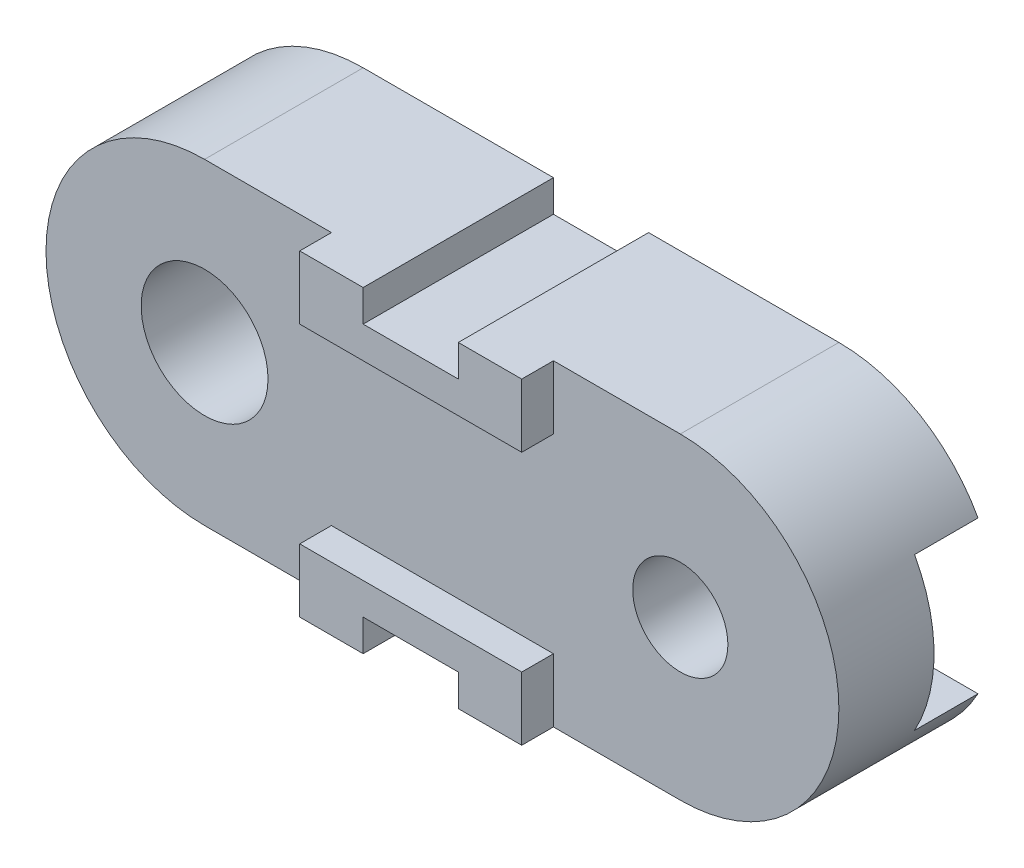
ISO-10303-21;
HEADER;
FILE_DESCRIPTION(('STEP AP214'),'2;1');
FILE_NAME('part.step','',(''),(''),'','','');
FILE_SCHEMA(('AUTOMOTIVE_DESIGN { 1 0 10303 214 1 1 1 1 }'));
ENDSEC;
DATA;
#1=APPLICATION_CONTEXT('core data for automotive mechanical design processes');
#2=APPLICATION_PROTOCOL_DEFINITION('international standard','automotive_design',2000,#1);
#3=PRODUCT_CONTEXT('',#1,'mechanical');
#4=PRODUCT('Part','Part','',(#3));
#5=PRODUCT_RELATED_PRODUCT_CATEGORY('part','',(#4));
#6=PRODUCT_DEFINITION_FORMATION('','',#4);
#7=PRODUCT_DEFINITION_CONTEXT('part definition',#1,'design');
#8=PRODUCT_DEFINITION('design','',#6,#7);
#9=PRODUCT_DEFINITION_SHAPE('','',#8);
#10=(LENGTH_UNIT() NAMED_UNIT(*) SI_UNIT(.MILLI.,.METRE.));
#11=(NAMED_UNIT(*) PLANE_ANGLE_UNIT() SI_UNIT($,.RADIAN.));
#12=(NAMED_UNIT(*) SI_UNIT($,.STERADIAN.) SOLID_ANGLE_UNIT());
#13=UNCERTAINTY_MEASURE_WITH_UNIT(LENGTH_MEASURE(1.E-05),#10,'distance_accuracy_value','');
#14=(GEOMETRIC_REPRESENTATION_CONTEXT(3) GLOBAL_UNCERTAINTY_ASSIGNED_CONTEXT((#13)) GLOBAL_UNIT_ASSIGNED_CONTEXT((#10,
#11,#12)) REPRESENTATION_CONTEXT('',''));
#15=CARTESIAN_POINT('',(0.,0.,0.));
#16=DIRECTION('',(0.,0.,1.));
#17=DIRECTION('',(1.,0.,0.));
#18=AXIS2_PLACEMENT_3D('',#15,#16,#17);
#19=CARTESIAN_POINT('',(-37.5,-25.,25.));
#20=DIRECTION('',(0.,1.,0.));
#21=DIRECTION('',(-1.,0.,0.));
#22=AXIS2_PLACEMENT_3D('',#19,#20,#21);
#23=PLANE('',#22);
#24=DIRECTION('',(1.,0.,0.));
#25=VECTOR('',#24,1.);
#26=CARTESIAN_POINT('',(17.5,-25.,30.));
#27=LINE('',#26,#25);
#28=CARTESIAN_POINT('',(7.5,-25.,30.));
#29=VERTEX_POINT('',#28);
#30=CARTESIAN_POINT('',(17.5,-25.,30.));
#31=VERTEX_POINT('',#30);
#32=EDGE_CURVE('E327',#29,#31,#27,.T.);
#33=ORIENTED_EDGE('',*,*,#32,.F.);
#34=DIRECTION('',(0.,0.,-1.));
#35=VECTOR('',#34,1.);
#36=CARTESIAN_POINT('',(7.5,-25.,25.));
#37=LINE('',#36,#35);
#38=CARTESIAN_POINT('',(7.5,-25.,0.));
#39=VERTEX_POINT('',#38);
#40=EDGE_CURVE('E281',#29,#39,#37,.T.);
#41=ORIENTED_EDGE('',*,*,#40,.T.);
#42=DIRECTION('',(1.,0.,0.));
#43=VECTOR('',#42,1.);
#44=CARTESIAN_POINT('',(-37.5,-25.,0.));
#45=LINE('',#44,#43);
#46=CARTESIAN_POINT('',(37.5,-25.,0.));
#47=VERTEX_POINT('',#46);
#48=EDGE_CURVE('E367',#39,#47,#45,.T.);
#49=ORIENTED_EDGE('',*,*,#48,.T.);
#50=DIRECTION('',(0.,0.,-1.));
#51=VECTOR('',#50,1.);
#52=CARTESIAN_POINT('',(37.5,-25.,25.));
#53=LINE('',#52,#51);
#54=CARTESIAN_POINT('',(37.5,-25.,25.));
#55=VERTEX_POINT('',#54);
#56=EDGE_CURVE('E387',#55,#47,#53,.T.);
#57=ORIENTED_EDGE('',*,*,#56,.F.);
#58=DIRECTION('',(1.,0.,0.));
#59=VECTOR('',#58,1.);
#60=CARTESIAN_POINT('',(-37.5,-25.,25.));
#61=LINE('',#60,#59);
#62=CARTESIAN_POINT('',(17.5,-25.,25.));
#63=VERTEX_POINT('',#62);
#64=EDGE_CURVE('E357',#63,#55,#61,.T.);
#65=ORIENTED_EDGE('',*,*,#64,.F.);
#66=DIRECTION('',(0.,0.,-1.));
#67=VECTOR('',#66,1.);
#68=CARTESIAN_POINT('',(17.5,-25.,30.));
#69=LINE('',#68,#67);
#70=EDGE_CURVE('E344',#31,#63,#69,.T.);
#71=ORIENTED_EDGE('',*,*,#70,.F.);
#72=EDGE_LOOP('',(#33,#41,#49,#57,#65,#71));
#73=FACE_BOUND('',#72,.T.);
#74=ADVANCED_FACE('F44',(#73),#23,.F.);
#75=CARTESIAN_POINT('',(-37.5,25.,25.));
#76=DIRECTION('',(0.,-1.,0.));
#77=DIRECTION('',(1.,0.,0.));
#78=AXIS2_PLACEMENT_3D('',#75,#76,#77);
#79=PLANE('',#78);
#80=DIRECTION('',(-1.,0.,0.));
#81=VECTOR('',#80,1.);
#82=CARTESIAN_POINT('',(17.5,25.,30.));
#83=LINE('',#82,#81);
#84=CARTESIAN_POINT('',(-7.5,25.,30.));
#85=VERTEX_POINT('',#84);
#86=CARTESIAN_POINT('',(-17.5,25.,30.));
#87=VERTEX_POINT('',#86);
#88=EDGE_CURVE('E296',#85,#87,#83,.T.);
#89=ORIENTED_EDGE('',*,*,#88,.F.);
#90=DIRECTION('',(0.,0.,-1.));
#91=VECTOR('',#90,1.);
#92=CARTESIAN_POINT('',(-7.5,25.,25.));
#93=LINE('',#92,#91);
#94=CARTESIAN_POINT('',(-7.5,25.,0.));
#95=VERTEX_POINT('',#94);
#96=EDGE_CURVE('E271',#85,#95,#93,.T.);
#97=ORIENTED_EDGE('',*,*,#96,.T.);
#98=DIRECTION('',(-1.,0.,0.));
#99=VECTOR('',#98,1.);
#100=CARTESIAN_POINT('',(-37.5,25.,0.));
#101=LINE('',#100,#99);
#102=CARTESIAN_POINT('',(-37.5,25.,0.));
#103=VERTEX_POINT('',#102);
#104=EDGE_CURVE('E378',#95,#103,#101,.T.);
#105=ORIENTED_EDGE('',*,*,#104,.T.);
#106=DIRECTION('',(0.,0.,-1.));
#107=VECTOR('',#106,1.);
#108=CARTESIAN_POINT('',(-37.5,25.,25.));
#109=LINE('',#108,#107);
#110=CARTESIAN_POINT('',(-37.5,25.,25.));
#111=VERTEX_POINT('',#110);
#112=EDGE_CURVE('E370',#111,#103,#109,.T.);
#113=ORIENTED_EDGE('',*,*,#112,.F.);
#114=DIRECTION('',(-1.,0.,0.));
#115=VECTOR('',#114,1.);
#116=CARTESIAN_POINT('',(-37.5,25.,25.));
#117=LINE('',#116,#115);
#118=CARTESIAN_POINT('',(-17.5,25.,25.));
#119=VERTEX_POINT('',#118);
#120=EDGE_CURVE('E365',#119,#111,#117,.T.);
#121=ORIENTED_EDGE('',*,*,#120,.F.);
#122=DIRECTION('',(0.,0.,-1.));
#123=VECTOR('',#122,1.);
#124=CARTESIAN_POINT('',(-17.5,25.,30.));
#125=LINE('',#124,#123);
#126=EDGE_CURVE('E305',#87,#119,#125,.T.);
#127=ORIENTED_EDGE('',*,*,#126,.F.);
#128=EDGE_LOOP('',(#89,#97,#105,#113,#121,#127));
#129=FACE_BOUND('',#128,.T.);
#130=ADVANCED_FACE('F417',(#129),#79,.F.);
#131=CARTESIAN_POINT('',(-37.5,0.,25.));
#132=DIRECTION('',(0.,0.,1.));
#133=DIRECTION('',(1.,0.,0.));
#134=AXIS2_PLACEMENT_3D('',#131,#132,#133);
#135=PLANE('',#134);
#136=CARTESIAN_POINT('',(37.5,0.,25.));
#137=DIRECTION('',(0.,0.,1.));
#138=DIRECTION('',(1.,0.,0.));
#139=AXIS2_PLACEMENT_3D('',#136,#137,#138);
#140=CIRCLE('',#139,7.5);
#141=CARTESIAN_POINT('',(45.,0.,25.));
#142=VERTEX_POINT('',#141);
#143=EDGE_CURVE('E408',#142,#142,#140,.T.);
#144=ORIENTED_EDGE('',*,*,#143,.F.);
#145=EDGE_LOOP('',(#144));
#146=FACE_BOUND('',#145,.T.);
#147=CARTESIAN_POINT('',(-37.5,0.,25.));
#148=DIRECTION('',(0.,0.,1.));
#149=DIRECTION('',(1.,0.,0.));
#150=AXIS2_PLACEMENT_3D('',#147,#148,#149);
#151=CIRCLE('',#150,10.);
#152=CARTESIAN_POINT('',(-27.5,0.,25.));
#153=VERTEX_POINT('',#152);
#154=EDGE_CURVE('E235',#153,#153,#151,.T.);
#155=ORIENTED_EDGE('',*,*,#154,.F.);
#156=EDGE_LOOP('',(#155));
#157=FACE_BOUND('',#156,.T.);
#158=DIRECTION('',(1.,0.,0.));
#159=VECTOR('',#158,1.);
#160=CARTESIAN_POINT('',(0.,15.,25.));
#161=LINE('',#160,#159);
#162=CARTESIAN_POINT('',(-17.5,15.,25.));
#163=VERTEX_POINT('',#162);
#164=CARTESIAN_POINT('',(17.5,15.,25.));
#165=VERTEX_POINT('',#164);
#166=EDGE_CURVE('E304',#163,#165,#161,.T.);
#167=ORIENTED_EDGE('',*,*,#166,.F.);
#168=DIRECTION('',(0.,-1.,0.));
#169=VECTOR('',#168,1.);
#170=CARTESIAN_POINT('',(-17.5,25.,25.));
#171=LINE('',#170,#169);
#172=EDGE_CURVE('E288',#119,#163,#171,.T.);
#173=ORIENTED_EDGE('',*,*,#172,.F.);
#174=ORIENTED_EDGE('',*,*,#120,.T.);
#175=CARTESIAN_POINT('',(-37.5,0.,25.));
#176=DIRECTION('',(0.,0.,1.));
#177=DIRECTION('',(1.,0.,0.));
#178=AXIS2_PLACEMENT_3D('',#175,#176,#177);
#179=CIRCLE('',#178,25.);
#180=CARTESIAN_POINT('',(-37.5,-25.,25.));
#181=VERTEX_POINT('',#180);
#182=EDGE_CURVE('E354',#111,#181,#179,.T.);
#183=ORIENTED_EDGE('',*,*,#182,.T.);
#184=CARTESIAN_POINT('',(-17.5,-25.,25.));
#185=VERTEX_POINT('',#184);
#186=EDGE_CURVE('E359',#181,#185,#61,.T.);
#187=ORIENTED_EDGE('',*,*,#186,.T.);
#188=DIRECTION('',(0.,-1.,0.));
#189=VECTOR('',#188,1.);
#190=CARTESIAN_POINT('',(-17.5,-25.,25.));
#191=LINE('',#190,#189);
#192=CARTESIAN_POINT('',(-17.5,-15.,25.));
#193=VERTEX_POINT('',#192);
#194=EDGE_CURVE('E321',#193,#185,#191,.T.);
#195=ORIENTED_EDGE('',*,*,#194,.F.);
#196=DIRECTION('',(-1.,0.,0.));
#197=VECTOR('',#196,1.);
#198=CARTESIAN_POINT('',(0.,-15.,25.));
#199=LINE('',#198,#197);
#200=CARTESIAN_POINT('',(17.5,-15.,25.));
#201=VERTEX_POINT('',#200);
#202=EDGE_CURVE('E326',#201,#193,#199,.T.);
#203=ORIENTED_EDGE('',*,*,#202,.F.);
#204=DIRECTION('',(0.,1.,0.));
#205=VECTOR('',#204,1.);
#206=CARTESIAN_POINT('',(17.5,-15.,25.));
#207=LINE('',#206,#205);
#208=EDGE_CURVE('E336',#63,#201,#207,.T.);
#209=ORIENTED_EDGE('',*,*,#208,.F.);
#210=ORIENTED_EDGE('',*,*,#64,.T.);
#211=CARTESIAN_POINT('',(37.5,0.,25.));
#212=DIRECTION('',(0.,0.,1.));
#213=DIRECTION('',(1.,0.,0.));
#214=AXIS2_PLACEMENT_3D('',#211,#212,#213);
#215=CIRCLE('',#214,25.);
#216=CARTESIAN_POINT('',(37.5,25.,25.));
#217=VERTEX_POINT('',#216);
#218=EDGE_CURVE('E362',#55,#217,#215,.T.);
#219=ORIENTED_EDGE('',*,*,#218,.T.);
#220=CARTESIAN_POINT('',(17.5,25.,25.));
#221=VERTEX_POINT('',#220);
#222=EDGE_CURVE('E364',#217,#221,#117,.T.);
#223=ORIENTED_EDGE('',*,*,#222,.T.);
#224=DIRECTION('',(0.,1.,0.));
#225=VECTOR('',#224,1.);
#226=CARTESIAN_POINT('',(17.5,15.,25.));
#227=LINE('',#226,#225);
#228=EDGE_CURVE('E294',#165,#221,#227,.T.);
#229=ORIENTED_EDGE('',*,*,#228,.F.);
#230=EDGE_LOOP('',(#167,#173,#174,#183,#187,#195,#203,#209,#210,#219,#223,#229));
#231=FACE_BOUND('',#230,.T.);
#232=ADVANCED_FACE('F413',(#146,#157,#231),#135,.T.);
#233=CARTESIAN_POINT('',(-37.5,0.,25.));
#234=DIRECTION('',(0.,0.,-1.));
#235=DIRECTION('',(-1.,0.,0.));
#236=AXIS2_PLACEMENT_3D('',#233,#234,#235);
#237=CYLINDRICAL_SURFACE('',#236,25.);
#238=CARTESIAN_POINT('',(-37.5,0.,0.));
#239=DIRECTION('',(0.,0.,1.));
#240=DIRECTION('',(1.,0.,0.));
#241=AXIS2_PLACEMENT_3D('',#238,#239,#240);
#242=CIRCLE('',#241,25.);
#243=CARTESIAN_POINT('',(-37.5,-25.,0.));
#244=VERTEX_POINT('',#243);
#245=EDGE_CURVE('E352',#103,#244,#242,.T.);
#246=ORIENTED_EDGE('',*,*,#245,.T.);
#247=DIRECTION('',(0.,0.,-1.));
#248=VECTOR('',#247,1.);
#249=CARTESIAN_POINT('',(-37.5,-25.,25.));
#250=LINE('',#249,#248);
#251=EDGE_CURVE('E386',#181,#244,#250,.T.);
#252=ORIENTED_EDGE('',*,*,#251,.F.);
#253=ORIENTED_EDGE('',*,*,#182,.F.);
#254=ORIENTED_EDGE('',*,*,#112,.T.);
#255=EDGE_LOOP('',(#246,#252,#253,#254));
#256=FACE_BOUND('',#255,.T.);
#257=ADVANCED_FACE('F50',(#256),#237,.T.);
#258=CARTESIAN_POINT('',(-7.5,-25.,0.));
#259=VERTEX_POINT('',#258);
#260=EDGE_CURVE('E371',#244,#259,#45,.T.);
#261=ORIENTED_EDGE('',*,*,#260,.T.);
#262=DIRECTION('',(0.,0.,1.));
#263=VECTOR('',#262,1.);
#264=CARTESIAN_POINT('',(-7.5,-25.,25.));
#265=LINE('',#264,#263);
#266=CARTESIAN_POINT('',(-7.5,-25.,30.));
#267=VERTEX_POINT('',#266);
#268=EDGE_CURVE('E280',#259,#267,#265,.T.);
#269=ORIENTED_EDGE('',*,*,#268,.T.);
#270=CARTESIAN_POINT('',(-17.5,-25.,30.));
#271=VERTEX_POINT('',#270);
#272=EDGE_CURVE('E328',#271,#267,#27,.T.);
#273=ORIENTED_EDGE('',*,*,#272,.F.);
#274=DIRECTION('',(0.,0.,-1.));
#275=VECTOR('',#274,1.);
#276=CARTESIAN_POINT('',(-17.5,-25.,30.));
#277=LINE('',#276,#275);
#278=EDGE_CURVE('E346',#271,#185,#277,.T.);
#279=ORIENTED_EDGE('',*,*,#278,.T.);
#280=ORIENTED_EDGE('',*,*,#186,.F.);
#281=ORIENTED_EDGE('',*,*,#251,.T.);
#282=EDGE_LOOP('',(#261,#269,#273,#279,#280,#281));
#283=FACE_BOUND('',#282,.T.);
#284=ADVANCED_FACE('F440',(#283),#23,.F.);
#285=CARTESIAN_POINT('',(37.5,0.,25.));
#286=DIRECTION('',(0.,0.,-1.));
#287=DIRECTION('',(-1.,0.,0.));
#288=AXIS2_PLACEMENT_3D('',#285,#286,#287);
#289=CYLINDRICAL_SURFACE('',#288,25.);
#290=CARTESIAN_POINT('',(37.5,0.,0.));
#291=DIRECTION('',(0.,0.,1.));
#292=DIRECTION('',(1.,0.,0.));
#293=AXIS2_PLACEMENT_3D('',#290,#291,#292);
#294=CIRCLE('',#293,25.);
#295=CARTESIAN_POINT('',(59.4317121994613,-12.,0.));
#296=VERTEX_POINT('',#295);
#297=EDGE_CURVE('E374',#47,#296,#294,.T.);
#298=ORIENTED_EDGE('',*,*,#297,.T.);
#299=DIRECTION('',(0.,0.,-1.));
#300=VECTOR('',#299,1.);
#301=CARTESIAN_POINT('',(59.4317121994613,-12.,25.));
#302=LINE('',#301,#300);
#303=CARTESIAN_POINT('',(59.4317121994613,-12.,10.));
#304=VERTEX_POINT('',#303);
#305=EDGE_CURVE('E238',#296,#304,#302,.F.);
#306=ORIENTED_EDGE('',*,*,#305,.T.);
#307=CARTESIAN_POINT('',(37.5,0.,10.));
#308=DIRECTION('',(0.,0.,-1.));
#309=DIRECTION('',(-1.,0.,0.));
#310=AXIS2_PLACEMENT_3D('',#307,#308,#309);
#311=CIRCLE('',#310,25.);
#312=CARTESIAN_POINT('',(59.4317121994613,12.,10.));
#313=VERTEX_POINT('',#312);
#314=EDGE_CURVE('E11',#313,#304,#311,.T.);
#315=ORIENTED_EDGE('',*,*,#314,.F.);
#316=DIRECTION('',(0.,0.,-1.));
#317=VECTOR('',#316,1.);
#318=CARTESIAN_POINT('',(59.4317121994613,12.,25.));
#319=LINE('',#318,#317);
#320=CARTESIAN_POINT('',(59.4317121994613,12.,0.));
#321=VERTEX_POINT('',#320);
#322=EDGE_CURVE('E222',#313,#321,#319,.T.);
#323=ORIENTED_EDGE('',*,*,#322,.T.);
#324=CARTESIAN_POINT('',(37.5,25.,0.));
#325=VERTEX_POINT('',#324);
#326=EDGE_CURVE('E372',#321,#325,#294,.T.);
#327=ORIENTED_EDGE('',*,*,#326,.T.);
#328=DIRECTION('',(0.,0.,-1.));
#329=VECTOR('',#328,1.);
#330=CARTESIAN_POINT('',(37.5,25.,25.));
#331=LINE('',#330,#329);
#332=EDGE_CURVE('E382',#217,#325,#331,.T.);
#333=ORIENTED_EDGE('',*,*,#332,.F.);
#334=ORIENTED_EDGE('',*,*,#218,.F.);
#335=ORIENTED_EDGE('',*,*,#56,.T.);
#336=EDGE_LOOP('',(#298,#306,#315,#323,#327,#333,#334,#335));
#337=FACE_BOUND('',#336,.T.);
#338=ADVANCED_FACE('F459',(#337),#289,.T.);
#339=CARTESIAN_POINT('',(7.5,25.,0.));
#340=VERTEX_POINT('',#339);
#341=EDGE_CURVE('E358',#325,#340,#101,.T.);
#342=ORIENTED_EDGE('',*,*,#341,.T.);
#343=DIRECTION('',(0.,0.,1.));
#344=VECTOR('',#343,1.);
#345=CARTESIAN_POINT('',(7.5,25.,25.));
#346=LINE('',#345,#344);
#347=CARTESIAN_POINT('',(7.5,25.,30.));
#348=VERTEX_POINT('',#347);
#349=EDGE_CURVE('E264',#340,#348,#346,.T.);
#350=ORIENTED_EDGE('',*,*,#349,.T.);
#351=CARTESIAN_POINT('',(17.5,25.,30.));
#352=VERTEX_POINT('',#351);
#353=EDGE_CURVE('E297',#352,#348,#83,.T.);
#354=ORIENTED_EDGE('',*,*,#353,.F.);
#355=DIRECTION('',(0.,0.,-1.));
#356=VECTOR('',#355,1.);
#357=CARTESIAN_POINT('',(17.5,25.,30.));
#358=LINE('',#357,#356);
#359=EDGE_CURVE('E315',#352,#221,#358,.T.);
#360=ORIENTED_EDGE('',*,*,#359,.T.);
#361=ORIENTED_EDGE('',*,*,#222,.F.);
#362=ORIENTED_EDGE('',*,*,#332,.T.);
#363=EDGE_LOOP('',(#342,#350,#354,#360,#361,#362));
#364=FACE_BOUND('',#363,.T.);
#365=ADVANCED_FACE('F470',(#364),#79,.F.);
#366=CARTESIAN_POINT('',(-37.5,0.,0.));
#367=DIRECTION('',(0.,0.,1.));
#368=DIRECTION('',(1.,0.,0.));
#369=AXIS2_PLACEMENT_3D('',#366,#367,#368);
#370=PLANE('',#369);
#371=CARTESIAN_POINT('',(-37.5,0.,0.));
#372=DIRECTION('',(0.,0.,1.));
#373=DIRECTION('',(1.,0.,0.));
#374=AXIS2_PLACEMENT_3D('',#371,#372,#373);
#375=CIRCLE('',#374,10.);
#376=CARTESIAN_POINT('',(-27.5,0.,0.));
#377=VERTEX_POINT('',#376);
#378=EDGE_CURVE('E237',#377,#377,#375,.T.);
#379=ORIENTED_EDGE('',*,*,#378,.T.);
#380=EDGE_LOOP('',(#379));
#381=FACE_BOUND('',#380,.T.);
#382=CARTESIAN_POINT('',(37.5,0.,0.));
#383=DIRECTION('',(0.,0.,-1.));
#384=DIRECTION('',(-1.,0.,0.));
#385=AXIS2_PLACEMENT_3D('',#382,#383,#384);
#386=CIRCLE('',#385,12.);
#387=CARTESIAN_POINT('',(37.5,-12.,0.));
#388=VERTEX_POINT('',#387);
#389=CARTESIAN_POINT('',(37.5,12.,0.));
#390=VERTEX_POINT('',#389);
#391=EDGE_CURVE('E65',#388,#390,#386,.T.);
#392=ORIENTED_EDGE('',*,*,#391,.F.);
#393=DIRECTION('',(1.,0.,0.));
#394=VECTOR('',#393,1.);
#395=CARTESIAN_POINT('',(-37.5,-12.,0.));
#396=LINE('',#395,#394);
#397=EDGE_CURVE('E53',#388,#296,#396,.T.);
#398=ORIENTED_EDGE('',*,*,#397,.T.);
#399=ORIENTED_EDGE('',*,*,#297,.F.);
#400=ORIENTED_EDGE('',*,*,#48,.F.);
#401=DIRECTION('',(0.,1.,0.));
#402=VECTOR('',#401,1.);
#403=CARTESIAN_POINT('',(7.5,0.,0.));
#404=LINE('',#403,#402);
#405=CARTESIAN_POINT('',(7.5,-20.,0.));
#406=VERTEX_POINT('',#405);
#407=EDGE_CURVE('E278',#39,#406,#404,.T.);
#408=ORIENTED_EDGE('',*,*,#407,.T.);
#409=DIRECTION('',(-1.,0.,0.));
#410=VECTOR('',#409,1.);
#411=CARTESIAN_POINT('',(-37.5,-20.,0.));
#412=LINE('',#411,#410);
#413=CARTESIAN_POINT('',(-7.5,-20.,0.));
#414=VERTEX_POINT('',#413);
#415=EDGE_CURVE('E286',#406,#414,#412,.T.);
#416=ORIENTED_EDGE('',*,*,#415,.T.);
#417=DIRECTION('',(0.,-1.,0.));
#418=VECTOR('',#417,1.);
#419=CARTESIAN_POINT('',(-7.5,0.,0.));
#420=LINE('',#419,#418);
#421=EDGE_CURVE('E273',#414,#259,#420,.T.);
#422=ORIENTED_EDGE('',*,*,#421,.T.);
#423=ORIENTED_EDGE('',*,*,#260,.F.);
#424=ORIENTED_EDGE('',*,*,#245,.F.);
#425=ORIENTED_EDGE('',*,*,#104,.F.);
#426=DIRECTION('',(0.,-1.,0.));
#427=VECTOR('',#426,1.);
#428=CARTESIAN_POINT('',(-7.5,0.,0.));
#429=LINE('',#428,#427);
#430=CARTESIAN_POINT('',(-7.5,20.,0.));
#431=VERTEX_POINT('',#430);
#432=EDGE_CURVE('E268',#95,#431,#429,.T.);
#433=ORIENTED_EDGE('',*,*,#432,.T.);
#434=DIRECTION('',(1.,0.,0.));
#435=VECTOR('',#434,1.);
#436=CARTESIAN_POINT('',(-37.5,20.,0.));
#437=LINE('',#436,#435);
#438=CARTESIAN_POINT('',(7.5,20.,0.));
#439=VERTEX_POINT('',#438);
#440=EDGE_CURVE('E253',#431,#439,#437,.T.);
#441=ORIENTED_EDGE('',*,*,#440,.T.);
#442=DIRECTION('',(0.,1.,0.));
#443=VECTOR('',#442,1.);
#444=CARTESIAN_POINT('',(7.5,0.,0.));
#445=LINE('',#444,#443);
#446=EDGE_CURVE('E265',#439,#340,#445,.T.);
#447=ORIENTED_EDGE('',*,*,#446,.T.);
#448=ORIENTED_EDGE('',*,*,#341,.F.);
#449=ORIENTED_EDGE('',*,*,#326,.F.);
#450=DIRECTION('',(1.,0.,0.));
#451=VECTOR('',#450,1.);
#452=CARTESIAN_POINT('',(37.5,12.,0.));
#453=LINE('',#452,#451);
#454=EDGE_CURVE('E226',#390,#321,#453,.T.);
#455=ORIENTED_EDGE('',*,*,#454,.F.);
#456=EDGE_LOOP('',(#392,#398,#399,#400,#408,#416,#422,#423,#424,#425,#433,#441,#447,#448,#449,#455));
#457=FACE_BOUND('',#456,.T.);
#458=ADVANCED_FACE('F476',(#381,#457),#370,.F.);
#459=CARTESIAN_POINT('',(-17.5,-25.,30.));
#460=DIRECTION('',(1.,0.,0.));
#461=DIRECTION('',(0.,0.,-1.));
#462=AXIS2_PLACEMENT_3D('',#459,#460,#461);
#463=PLANE('',#462);
#464=ORIENTED_EDGE('',*,*,#194,.T.);
#465=ORIENTED_EDGE('',*,*,#278,.F.);
#466=DIRECTION('',(0.,-1.,0.));
#467=VECTOR('',#466,1.);
#468=CARTESIAN_POINT('',(-17.5,-25.,30.));
#469=LINE('',#468,#467);
#470=CARTESIAN_POINT('',(-17.5,-15.,30.));
#471=VERTEX_POINT('',#470);
#472=EDGE_CURVE('E324',#471,#271,#469,.T.);
#473=ORIENTED_EDGE('',*,*,#472,.F.);
#474=DIRECTION('',(0.,0.,-1.));
#475=VECTOR('',#474,1.);
#476=CARTESIAN_POINT('',(-17.5,-15.,30.));
#477=LINE('',#476,#475);
#478=EDGE_CURVE('E353',#471,#193,#477,.T.);
#479=ORIENTED_EDGE('',*,*,#478,.T.);
#480=EDGE_LOOP('',(#464,#465,#473,#479));
#481=FACE_BOUND('',#480,.T.);
#482=ADVANCED_FACE('F442',(#481),#463,.F.);
#483=CARTESIAN_POINT('',(17.5,-15.,30.));
#484=DIRECTION('',(-1.,0.,0.));
#485=DIRECTION('',(0.,0.,1.));
#486=AXIS2_PLACEMENT_3D('',#483,#484,#485);
#487=PLANE('',#486);
#488=ORIENTED_EDGE('',*,*,#208,.T.);
#489=DIRECTION('',(0.,0.,-1.));
#490=VECTOR('',#489,1.);
#491=CARTESIAN_POINT('',(17.5,-15.,30.));
#492=LINE('',#491,#490);
#493=CARTESIAN_POINT('',(17.5,-15.,30.));
#494=VERTEX_POINT('',#493);
#495=EDGE_CURVE('E333',#494,#201,#492,.T.);
#496=ORIENTED_EDGE('',*,*,#495,.F.);
#497=DIRECTION('',(0.,1.,0.));
#498=VECTOR('',#497,1.);
#499=CARTESIAN_POINT('',(17.5,-15.,30.));
#500=LINE('',#499,#498);
#501=EDGE_CURVE('E335',#31,#494,#500,.T.);
#502=ORIENTED_EDGE('',*,*,#501,.F.);
#503=ORIENTED_EDGE('',*,*,#70,.T.);
#504=EDGE_LOOP('',(#488,#496,#502,#503));
#505=FACE_BOUND('',#504,.T.);
#506=ADVANCED_FACE('F446',(#505),#487,.F.);
#507=CARTESIAN_POINT('',(0.,-15.,30.));
#508=DIRECTION('',(0.,-1.,0.));
#509=DIRECTION('',(0.,0.,-1.));
#510=AXIS2_PLACEMENT_3D('',#507,#508,#509);
#511=PLANE('',#510);
#512=ORIENTED_EDGE('',*,*,#202,.T.);
#513=ORIENTED_EDGE('',*,*,#478,.F.);
#514=DIRECTION('',(-1.,0.,0.));
#515=VECTOR('',#514,1.);
#516=CARTESIAN_POINT('',(-17.5,-15.,30.));
#517=LINE('',#516,#515);
#518=EDGE_CURVE('E325',#494,#471,#517,.T.);
#519=ORIENTED_EDGE('',*,*,#518,.F.);
#520=ORIENTED_EDGE('',*,*,#495,.T.);
#521=EDGE_LOOP('',(#512,#513,#519,#520));
#522=FACE_BOUND('',#521,.T.);
#523=ADVANCED_FACE('F441',(#522),#511,.F.);
#524=CARTESIAN_POINT('',(0.,0.,30.));
#525=DIRECTION('',(0.,0.,-1.));
#526=DIRECTION('',(-1.,0.,0.));
#527=AXIS2_PLACEMENT_3D('',#524,#525,#526);
#528=PLANE('',#527);
#529=DIRECTION('',(-1.,0.,0.));
#530=VECTOR('',#529,1.);
#531=CARTESIAN_POINT('',(0.,-20.,30.));
#532=LINE('',#531,#530);
#533=CARTESIAN_POINT('',(7.5,-20.,30.));
#534=VERTEX_POINT('',#533);
#535=CARTESIAN_POINT('',(-7.5,-20.,30.));
#536=VERTEX_POINT('',#535);
#537=EDGE_CURVE('E69',#534,#536,#532,.T.);
#538=ORIENTED_EDGE('',*,*,#537,.F.);
#539=DIRECTION('',(0.,-1.,0.));
#540=VECTOR('',#539,1.);
#541=CARTESIAN_POINT('',(7.5,0.,30.));
#542=LINE('',#541,#540);
#543=EDGE_CURVE('E394',#534,#29,#542,.T.);
#544=ORIENTED_EDGE('',*,*,#543,.T.);
#545=ORIENTED_EDGE('',*,*,#32,.T.);
#546=ORIENTED_EDGE('',*,*,#501,.T.);
#547=ORIENTED_EDGE('',*,*,#518,.T.);
#548=ORIENTED_EDGE('',*,*,#472,.T.);
#549=ORIENTED_EDGE('',*,*,#272,.T.);
#550=DIRECTION('',(0.,-1.,0.));
#551=VECTOR('',#550,1.);
#552=CARTESIAN_POINT('',(-7.5,-26.5386541931155,30.));
#553=LINE('',#552,#551);
#554=EDGE_CURVE('E242',#536,#267,#553,.T.);
#555=ORIENTED_EDGE('',*,*,#554,.F.);
#556=EDGE_LOOP('',(#538,#544,#545,#546,#547,#548,#549,#555));
#557=FACE_BOUND('',#556,.T.);
#558=ADVANCED_FACE('F542',(#557),#528,.F.);
#559=CARTESIAN_POINT('',(-17.5,25.,30.));
#560=DIRECTION('',(1.,0.,0.));
#561=DIRECTION('',(0.,0.,-1.));
#562=AXIS2_PLACEMENT_3D('',#559,#560,#561);
#563=PLANE('',#562);
#564=ORIENTED_EDGE('',*,*,#172,.T.);
#565=DIRECTION('',(0.,0.,-1.));
#566=VECTOR('',#565,1.);
#567=CARTESIAN_POINT('',(-17.5,15.,30.));
#568=LINE('',#567,#566);
#569=CARTESIAN_POINT('',(-17.5,15.,30.));
#570=VERTEX_POINT('',#569);
#571=EDGE_CURVE('E318',#570,#163,#568,.T.);
#572=ORIENTED_EDGE('',*,*,#571,.F.);
#573=DIRECTION('',(0.,-1.,0.));
#574=VECTOR('',#573,1.);
#575=CARTESIAN_POINT('',(-17.5,25.,30.));
#576=LINE('',#575,#574);
#577=EDGE_CURVE('E289',#87,#570,#576,.T.);
#578=ORIENTED_EDGE('',*,*,#577,.F.);
#579=ORIENTED_EDGE('',*,*,#126,.T.);
#580=EDGE_LOOP('',(#564,#572,#578,#579));
#581=FACE_BOUND('',#580,.T.);
#582=ADVANCED_FACE('F430',(#581),#563,.F.);
#583=CARTESIAN_POINT('',(0.,15.,30.));
#584=DIRECTION('',(0.,1.,0.));
#585=DIRECTION('',(0.,0.,1.));
#586=AXIS2_PLACEMENT_3D('',#583,#584,#585);
#587=PLANE('',#586);
#588=ORIENTED_EDGE('',*,*,#166,.T.);
#589=DIRECTION('',(0.,0.,-1.));
#590=VECTOR('',#589,1.);
#591=CARTESIAN_POINT('',(17.5,15.,30.));
#592=LINE('',#591,#590);
#593=CARTESIAN_POINT('',(17.5,15.,30.));
#594=VERTEX_POINT('',#593);
#595=EDGE_CURVE('E312',#594,#165,#592,.T.);
#596=ORIENTED_EDGE('',*,*,#595,.F.);
#597=DIRECTION('',(1.,0.,0.));
#598=VECTOR('',#597,1.);
#599=CARTESIAN_POINT('',(-17.5,15.,30.));
#600=LINE('',#599,#598);
#601=EDGE_CURVE('E291',#570,#594,#600,.T.);
#602=ORIENTED_EDGE('',*,*,#601,.F.);
#603=ORIENTED_EDGE('',*,*,#571,.T.);
#604=EDGE_LOOP('',(#588,#596,#602,#603));
#605=FACE_BOUND('',#604,.T.);
#606=ADVANCED_FACE('F424',(#605),#587,.F.);
#607=CARTESIAN_POINT('',(17.5,15.,30.));
#608=DIRECTION('',(-1.,0.,0.));
#609=DIRECTION('',(0.,0.,1.));
#610=AXIS2_PLACEMENT_3D('',#607,#608,#609);
#611=PLANE('',#610);
#612=ORIENTED_EDGE('',*,*,#228,.T.);
#613=ORIENTED_EDGE('',*,*,#359,.F.);
#614=DIRECTION('',(0.,1.,0.));
#615=VECTOR('',#614,1.);
#616=CARTESIAN_POINT('',(17.5,15.,30.));
#617=LINE('',#616,#615);
#618=EDGE_CURVE('E298',#594,#352,#617,.T.);
#619=ORIENTED_EDGE('',*,*,#618,.F.);
#620=ORIENTED_EDGE('',*,*,#595,.T.);
#621=EDGE_LOOP('',(#612,#613,#619,#620));
#622=FACE_BOUND('',#621,.T.);
#623=ADVANCED_FACE('F462',(#622),#611,.F.);
#624=CARTESIAN_POINT('',(0.,0.,30.));
#625=DIRECTION('',(0.,0.,1.));
#626=DIRECTION('',(1.,0.,0.));
#627=AXIS2_PLACEMENT_3D('',#624,#625,#626);
#628=PLANE('',#627);
#629=DIRECTION('',(0.,-1.,0.));
#630=VECTOR('',#629,1.);
#631=CARTESIAN_POINT('',(-7.5,0.,30.));
#632=LINE('',#631,#630);
#633=CARTESIAN_POINT('',(-7.5,20.,30.));
#634=VERTEX_POINT('',#633);
#635=EDGE_CURVE('E395',#85,#634,#632,.T.);
#636=ORIENTED_EDGE('',*,*,#635,.F.);
#637=ORIENTED_EDGE('',*,*,#88,.T.);
#638=ORIENTED_EDGE('',*,*,#577,.T.);
#639=ORIENTED_EDGE('',*,*,#601,.T.);
#640=ORIENTED_EDGE('',*,*,#618,.T.);
#641=ORIENTED_EDGE('',*,*,#353,.T.);
#642=DIRECTION('',(0.,1.,0.));
#643=VECTOR('',#642,1.);
#644=CARTESIAN_POINT('',(7.5,20.,30.));
#645=LINE('',#644,#643);
#646=CARTESIAN_POINT('',(7.5,20.,30.));
#647=VERTEX_POINT('',#646);
#648=EDGE_CURVE('E254',#647,#348,#645,.T.);
#649=ORIENTED_EDGE('',*,*,#648,.F.);
#650=DIRECTION('',(1.,0.,0.));
#651=VECTOR('',#650,1.);
#652=CARTESIAN_POINT('',(0.,20.,30.));
#653=LINE('',#652,#651);
#654=EDGE_CURVE('E241',#634,#647,#653,.T.);
#655=ORIENTED_EDGE('',*,*,#654,.F.);
#656=EDGE_LOOP('',(#636,#637,#638,#639,#640,#641,#649,#655));
#657=FACE_BOUND('',#656,.T.);
#658=ADVANCED_FACE('F473',(#657),#628,.T.);
#659=CARTESIAN_POINT('',(-7.5,26.5386541931155,-5.));
#660=DIRECTION('',(-1.,0.,0.));
#661=DIRECTION('',(0.,0.,1.));
#662=AXIS2_PLACEMENT_3D('',#659,#660,#661);
#663=PLANE('',#662);
#664=ORIENTED_EDGE('',*,*,#635,.T.);
#665=DIRECTION('',(0.,0.,1.));
#666=VECTOR('',#665,1.);
#667=CARTESIAN_POINT('',(-7.5,20.,-5.));
#668=LINE('',#667,#666);
#669=EDGE_CURVE('E260',#431,#634,#668,.T.);
#670=ORIENTED_EDGE('',*,*,#669,.F.);
#671=ORIENTED_EDGE('',*,*,#432,.F.);
#672=ORIENTED_EDGE('',*,*,#96,.F.);
#673=EDGE_LOOP('',(#664,#670,#671,#672));
#674=FACE_BOUND('',#673,.T.);
#675=ADVANCED_FACE('F474',(#674),#663,.F.);
#676=CARTESIAN_POINT('',(7.5,20.,-5.));
#677=DIRECTION('',(1.,0.,0.));
#678=DIRECTION('',(0.,0.,-1.));
#679=AXIS2_PLACEMENT_3D('',#676,#677,#678);
#680=PLANE('',#679);
#681=ORIENTED_EDGE('',*,*,#446,.F.);
#682=DIRECTION('',(0.,0.,1.));
#683=VECTOR('',#682,1.);
#684=CARTESIAN_POINT('',(7.5,20.,-5.));
#685=LINE('',#684,#683);
#686=EDGE_CURVE('E246',#439,#647,#685,.T.);
#687=ORIENTED_EDGE('',*,*,#686,.T.);
#688=ORIENTED_EDGE('',*,*,#648,.T.);
#689=ORIENTED_EDGE('',*,*,#349,.F.);
#690=EDGE_LOOP('',(#681,#687,#688,#689));
#691=FACE_BOUND('',#690,.T.);
#692=ADVANCED_FACE('F492',(#691),#680,.F.);
#693=CARTESIAN_POINT('',(0.,20.,-5.));
#694=DIRECTION('',(0.,-1.,0.));
#695=DIRECTION('',(0.,0.,-1.));
#696=AXIS2_PLACEMENT_3D('',#693,#694,#695);
#697=PLANE('',#696);
#698=ORIENTED_EDGE('',*,*,#669,.T.);
#699=ORIENTED_EDGE('',*,*,#654,.T.);
#700=ORIENTED_EDGE('',*,*,#686,.F.);
#701=ORIENTED_EDGE('',*,*,#440,.F.);
#702=EDGE_LOOP('',(#698,#699,#700,#701));
#703=FACE_BOUND('',#702,.T.);
#704=ADVANCED_FACE('F494',(#703),#697,.F.);
#705=CARTESIAN_POINT('',(0.,-20.,-5.));
#706=DIRECTION('',(0.,1.,0.));
#707=DIRECTION('',(0.,0.,1.));
#708=AXIS2_PLACEMENT_3D('',#705,#706,#707);
#709=PLANE('',#708);
#710=DIRECTION('',(0.,0.,1.));
#711=VECTOR('',#710,1.);
#712=CARTESIAN_POINT('',(7.5,-20.,-5.));
#713=LINE('',#712,#711);
#714=EDGE_CURVE('E248',#406,#534,#713,.T.);
#715=ORIENTED_EDGE('',*,*,#714,.T.);
#716=ORIENTED_EDGE('',*,*,#537,.T.);
#717=DIRECTION('',(0.,0.,1.));
#718=VECTOR('',#717,1.);
#719=CARTESIAN_POINT('',(-7.5,-20.,-5.));
#720=LINE('',#719,#718);
#721=EDGE_CURVE('E247',#414,#536,#720,.T.);
#722=ORIENTED_EDGE('',*,*,#721,.F.);
#723=ORIENTED_EDGE('',*,*,#415,.F.);
#724=EDGE_LOOP('',(#715,#716,#722,#723));
#725=FACE_BOUND('',#724,.T.);
#726=ADVANCED_FACE('F485',(#725),#709,.F.);
#727=CARTESIAN_POINT('',(7.5,-20.,-5.));
#728=DIRECTION('',(1.,0.,0.));
#729=DIRECTION('',(0.,0.,-1.));
#730=AXIS2_PLACEMENT_3D('',#727,#728,#729);
#731=PLANE('',#730);
#732=ORIENTED_EDGE('',*,*,#543,.F.);
#733=ORIENTED_EDGE('',*,*,#714,.F.);
#734=ORIENTED_EDGE('',*,*,#407,.F.);
#735=ORIENTED_EDGE('',*,*,#40,.F.);
#736=EDGE_LOOP('',(#732,#733,#734,#735));
#737=FACE_BOUND('',#736,.T.);
#738=ADVANCED_FACE('F486',(#737),#731,.F.);
#739=CARTESIAN_POINT('',(-7.5,-26.5386541931155,-5.));
#740=DIRECTION('',(-1.,0.,0.));
#741=DIRECTION('',(0.,0.,1.));
#742=AXIS2_PLACEMENT_3D('',#739,#740,#741);
#743=PLANE('',#742);
#744=ORIENTED_EDGE('',*,*,#421,.F.);
#745=ORIENTED_EDGE('',*,*,#721,.T.);
#746=ORIENTED_EDGE('',*,*,#554,.T.);
#747=ORIENTED_EDGE('',*,*,#268,.F.);
#748=EDGE_LOOP('',(#744,#745,#746,#747));
#749=FACE_BOUND('',#748,.T.);
#750=ADVANCED_FACE('F477',(#749),#743,.F.);
#751=CARTESIAN_POINT('',(37.5,0.,10.));
#752=DIRECTION('',(0.,0.,-1.));
#753=DIRECTION('',(-1.,0.,0.));
#754=AXIS2_PLACEMENT_3D('',#751,#752,#753);
#755=PLANE('',#754);
#756=CARTESIAN_POINT('',(37.5,0.,10.));
#757=DIRECTION('',(0.,0.,-1.));
#758=DIRECTION('',(-1.,0.,0.));
#759=AXIS2_PLACEMENT_3D('',#756,#757,#758);
#760=CIRCLE('',#759,7.5);
#761=CARTESIAN_POINT('',(30.,0.,10.));
#762=VERTEX_POINT('',#761);
#763=EDGE_CURVE('E47',#762,#762,#760,.T.);
#764=ORIENTED_EDGE('',*,*,#763,.F.);
#765=EDGE_LOOP('',(#764));
#766=FACE_BOUND('',#765,.T.);
#767=ORIENTED_EDGE('',*,*,#314,.T.);
#768=DIRECTION('',(-1.,0.,0.));
#769=VECTOR('',#768,1.);
#770=CARTESIAN_POINT('',(37.5,-12.,10.));
#771=LINE('',#770,#769);
#772=CARTESIAN_POINT('',(37.5,-12.,10.));
#773=VERTEX_POINT('',#772);
#774=EDGE_CURVE('E214',#304,#773,#771,.T.);
#775=ORIENTED_EDGE('',*,*,#774,.T.);
#776=CARTESIAN_POINT('',(37.5,0.,10.));
#777=DIRECTION('',(0.,0.,-1.));
#778=DIRECTION('',(-1.,0.,0.));
#779=AXIS2_PLACEMENT_3D('',#776,#777,#778);
#780=CIRCLE('',#779,12.);
#781=CARTESIAN_POINT('',(37.5,12.,10.));
#782=VERTEX_POINT('',#781);
#783=EDGE_CURVE('E211',#773,#782,#780,.T.);
#784=ORIENTED_EDGE('',*,*,#783,.T.);
#785=DIRECTION('',(1.,0.,0.));
#786=VECTOR('',#785,1.);
#787=CARTESIAN_POINT('',(37.5,12.,10.));
#788=LINE('',#787,#786);
#789=EDGE_CURVE('E217',#782,#313,#788,.T.);
#790=ORIENTED_EDGE('',*,*,#789,.T.);
#791=EDGE_LOOP('',(#767,#775,#784,#790));
#792=FACE_BOUND('',#791,.T.);
#793=ADVANCED_FACE('F223',(#766,#792),#755,.T.);
#794=CARTESIAN_POINT('',(37.5,-12.,10.));
#795=DIRECTION('',(0.,-1.,0.));
#796=DIRECTION('',(0.,0.,-1.));
#797=AXIS2_PLACEMENT_3D('',#794,#795,#796);
#798=PLANE('',#797);
#799=ORIENTED_EDGE('',*,*,#397,.F.);
#800=DIRECTION('',(0.,0.,-1.));
#801=VECTOR('',#800,1.);
#802=CARTESIAN_POINT('',(37.5,-12.,10.));
#803=LINE('',#802,#801);
#804=EDGE_CURVE('E212',#773,#388,#803,.T.);
#805=ORIENTED_EDGE('',*,*,#804,.F.);
#806=ORIENTED_EDGE('',*,*,#774,.F.);
#807=ORIENTED_EDGE('',*,*,#305,.F.);
#808=EDGE_LOOP('',(#799,#805,#806,#807));
#809=FACE_BOUND('',#808,.T.);
#810=ADVANCED_FACE('F488',(#809),#798,.F.);
#811=CARTESIAN_POINT('',(37.5,12.,10.));
#812=DIRECTION('',(0.,1.,0.));
#813=DIRECTION('',(0.,0.,1.));
#814=AXIS2_PLACEMENT_3D('',#811,#812,#813);
#815=PLANE('',#814);
#816=ORIENTED_EDGE('',*,*,#789,.F.);
#817=DIRECTION('',(0.,0.,-1.));
#818=VECTOR('',#817,1.);
#819=CARTESIAN_POINT('',(37.5,12.,10.));
#820=LINE('',#819,#818);
#821=EDGE_CURVE('E210',#782,#390,#820,.T.);
#822=ORIENTED_EDGE('',*,*,#821,.T.);
#823=ORIENTED_EDGE('',*,*,#454,.T.);
#824=ORIENTED_EDGE('',*,*,#322,.F.);
#825=EDGE_LOOP('',(#816,#822,#823,#824));
#826=FACE_BOUND('',#825,.T.);
#827=ADVANCED_FACE('F218',(#826),#815,.F.);
#828=CARTESIAN_POINT('',(37.5,0.,10.));
#829=DIRECTION('',(0.,0.,-1.));
#830=DIRECTION('',(-1.,0.,0.));
#831=AXIS2_PLACEMENT_3D('',#828,#829,#830);
#832=CYLINDRICAL_SURFACE('',#831,12.);
#833=ORIENTED_EDGE('',*,*,#391,.T.);
#834=ORIENTED_EDGE('',*,*,#821,.F.);
#835=ORIENTED_EDGE('',*,*,#783,.F.);
#836=ORIENTED_EDGE('',*,*,#804,.T.);
#837=EDGE_LOOP('',(#833,#834,#835,#836));
#838=FACE_BOUND('',#837,.T.);
#839=ADVANCED_FACE('F207',(#838),#832,.F.);
#840=CARTESIAN_POINT('',(-37.5,0.,-7.));
#841=DIRECTION('',(0.,0.,1.));
#842=DIRECTION('',(1.,0.,0.));
#843=AXIS2_PLACEMENT_3D('',#840,#841,#842);
#844=CYLINDRICAL_SURFACE('',#843,10.);
#845=ORIENTED_EDGE('',*,*,#154,.T.);
#846=EDGE_LOOP('',(#845));
#847=FACE_BOUND('',#846,.T.);
#848=ORIENTED_EDGE('',*,*,#378,.F.);
#849=EDGE_LOOP('',(#848));
#850=FACE_BOUND('',#849,.T.);
#851=ADVANCED_FACE('F671',(#847,#850),#844,.F.);
#852=CARTESIAN_POINT('',(37.5,0.,-7.));
#853=DIRECTION('',(0.,0.,1.));
#854=DIRECTION('',(1.,0.,0.));
#855=AXIS2_PLACEMENT_3D('',#852,#853,#854);
#856=CYLINDRICAL_SURFACE('',#855,7.5);
#857=ORIENTED_EDGE('',*,*,#763,.T.);
#858=EDGE_LOOP('',(#857));
#859=FACE_BOUND('',#858,.T.);
#860=ORIENTED_EDGE('',*,*,#143,.T.);
#861=EDGE_LOOP('',(#860));
#862=FACE_BOUND('',#861,.T.);
#863=ADVANCED_FACE('F415',(#859,#862),#856,.F.);
#864=CLOSED_SHELL('',(#74,#130,#232,#257,#284,#338,#365,#458,#482,#506,#523,#558,#582,#606,#623,
#658,#675,#692,#704,#726,#738,#750,#793,#810,#827,#839,#851,#863));
#865=MANIFOLD_SOLID_BREP('B2',#864);
#866=ADVANCED_BREP_SHAPE_REPRESENTATION('',(#18,#865),#14);
#867=SHAPE_DEFINITION_REPRESENTATION(#9,#866);
ENDSEC;
END-ISO-10303-21;
